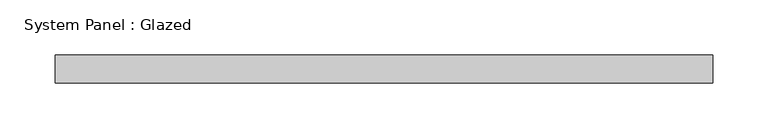
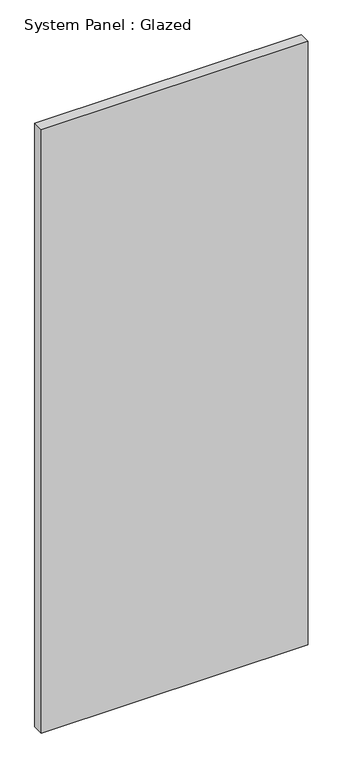
"""IFC4 building model written with IfcOpenShell, lengths in millimetres: plate geometry, System Panel : Glazed."""

from ifc_helpers import new_model, si_unit, origin, origin_with_axes, place, context, project, spatial, polyline, outline, extrude, source, transform, mapped, element, save


def system_panel_glazed_1c6e9dc7(model_context):
    return source(origin(), model_context, "Body", "SweptSolid", [
        extrude(outline(polyline([(298.45, 19.05), (-298.45, 19.05), (-298.45, 44.45), (298.45, 44.45), (298.45, 19.05)])), origin_with_axes(), (0.0, 0.0, 1.0), 1426.4572054),
    ])


if __name__ == "__main__":
    model = new_model("IFC4")
    model_context = context("Model", 3, world=origin())
    ifc_project = project(units=[si_unit("LENGTHUNIT", "METRE", prefix="MILLI")], contexts=[model_context])
    site = spatial("IfcSite", under=ifc_project)
    building = spatial("IfcBuilding", under=site)
    placement = place(None, origin())
    system_panel_glazed_shape = system_panel_glazed_1c6e9dc7(model_context)
    element("IfcPlate", 1, ObjectType="System Panel : Glazed", at=placement, inside=building, context=model_context, shape_type="MappedRepresentation", body=[
        mapped(system_panel_glazed_shape, transform((0.0, 0.0, 0.0), x_axis=(1.0, 0.0, 0.0), y_axis=(0.0, 1.0, 0.0), z_axis=(0.0, 0.0, 1.0))),
    ])
    save(model, "model.ifc")

# Revit data of these elements
# Type "System Panel : Glazed"
#   Construction Type Id = "GSP4R"
#   Analytic Construction = "1/8 in Pilkington single glazing"
#   Visual Light Transmittance = 0.9
#   Solar Heat Gain Coefficient = 0.86
#   Heat Transfer Coefficient (U) = 1.18115 BTU/(h·ft²·°F)
#   Define Thermal Properties by = 1
# Element 1 (IfcPlate, "System Panel : Glazed")
#   Materials on its faces: "Glass"
# Materials
#   "Glass": class "Glass", colour RGB 0 128 192, transparency 0.75, Description = "Soda Lime Glass", Cost = 0
